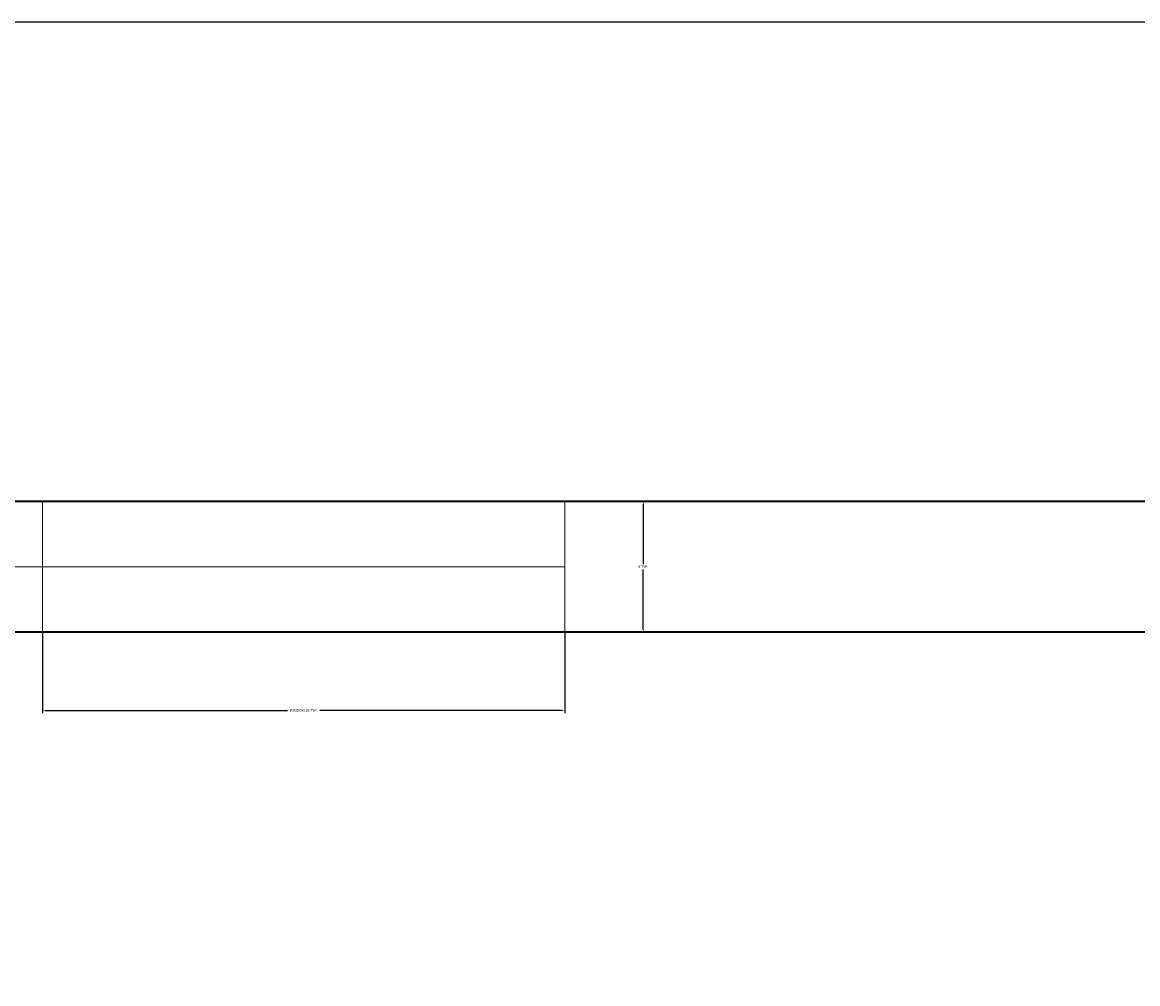
# Model space of a CAD drawing. Units: millimetres. Extents: x 27017497 to 27018854, y 7058029 to 7059154.
# Tile 46 of 91: x 27017673 to 27017750, y 7058557 to 7058623. Entities that reach past the tile are written whole.
import ezdxf

# ---------------------------------------------------------------- set-up
doc = ezdxf.new("R2010")
doc.units = ezdxf.units.MM
for name, color, linetype, lineweight in [('A-ANNO-DIMS', 2, 'Continuous', 18), ('A-GLAZ', 4, 'Continuous', 18), ('A-WALL', 7, 'Continuous', 35)]:
    doc.layers.add(name, color=color, linetype=linetype, lineweight=lineweight)
doc.styles.get("Standard").update_dxf_attribs({"font": 'arial.ttf'})
doc.dimstyles.get("Standard").update_dxf_attribs({"dimtxt": 0.18, "dimasz": 0.18, "dimexe": 0.18, "dimexo": 0.0625, "dimgap": 0.09, "dimtad": 0, "dimtih": 1, "dimtoh": 1, "dimdec": 4, "dimzin": 0, "dimdsep": 46, "dimtxsty": 'Standard', "dimcen": 0.09, "dimadec": 0, "dimazin": 0, "dimtfac": 1, "dimtdec": 4, "dimtofl": 0, "dimtmove": 0, "dimatfit": 3, "dimfxl": 1, "dimtolj": 1, "dimtzin": 0, "dimarcsym": 0})

# ---------------------------------------------------------------- blocks, each defined once
blk = doc.blocks.new('WINDOW-SINGLE-LIGHT')
blk.add_lwpolyline([(36, 4.5), (36, 0), (0, 0), (0, 9), (36, 9), (36, 4.5), (0, 4.5)])
blk = doc.blocks.new('*D19')
at = {"layer": 'A-ANNO-DIMS', "color": 0, "lineweight": -2, "transparency": 16777216}
for p, q in [((27017674.681, 7058580.826), (27017674.681, 7058575.309)), ((27017710.681, 7058580.826), (27017710.681, 7058575.309)), ((27017674.861, 7058575.489), (27017691.563, 7058575.489)), ((27017710.501, 7058575.489), (27017693.8, 7058575.489))]:
    blk.add_line(p, q, dxfattribs=at)
at = {"layer": 'A-ANNO-DIMS', "color": 0, "transparency": 16777216}
for points in [[(27017674.861, 7058575.519), (27017674.861, 7058575.459), (27017674.681, 7058575.489)], [(27017710.501, 7058575.519), (27017710.501, 7058575.459), (27017710.681, 7058575.489)]]:
    blk.add_solid(points, dxfattribs=at)
at = {"layer": 'Defpoints', "color": 0, "transparency": 16777216}
for p in [(27017674.681, 7058580.889), (27017710.681, 7058580.889), (27017710.681, 7058575.489)]:
    blk.add_point(p, dxfattribs=at)
at = {"layer": 'A-ANNO-DIMS', "color": 0, "transparency": 16777216, "insert": (27017692.681, 7058575.489), "char_height": 0.18, "attachment_point": 5}
blk.add_mtext('\\A1;WINDOW 36 TYP.', dxfattribs=at)
blk = doc.blocks.new('*D20')
at = {"layer": 'A-ANNO-DIMS', "color": 0, "lineweight": -2, "transparency": 16777216}
for p, q in [((27017710.744, 7058589.889), (27017716.261, 7058589.889)), ((27017716.081, 7058589.709), (27017716.081, 7058585.571)), ((27017716.081, 7058581.069), (27017716.081, 7058585.207)), ((27017710.744, 7058580.889), (27017716.261, 7058580.889))]:
    blk.add_line(p, q, dxfattribs=at)
at = {"layer": 'A-ANNO-DIMS', "color": 0, "transparency": 16777216}
for points in [[(27017716.051, 7058589.709), (27017716.111, 7058589.709), (27017716.081, 7058589.889)], [(27017716.051, 7058581.069), (27017716.111, 7058581.069), (27017716.081, 7058580.889)]]:
    blk.add_solid(points, dxfattribs=at)
at = {"layer": 'Defpoints', "color": 0, "transparency": 16777216}
for p in [(27017710.681, 7058589.889), (27017716.081, 7058589.889), (27017710.681, 7058580.889)]:
    blk.add_point(p, dxfattribs=at)
at = {"layer": 'A-ANNO-DIMS', "color": 0, "transparency": 16777216, "insert": (27017716.081, 7058585.389), "char_height": 0.18, "attachment_point": 5}
blk.add_mtext('\\A1;9 TYP.', dxfattribs=at)
blk = doc.blocks.new('*D48')
at = {"layer": 'A-ANNO-DIMS', "color": 0, "lineweight": -2, "transparency": 16777216}
for p, q in [((27018463.498, 7058622.912), (27017497.536, 7058622.912)), ((27017497.716, 7058622.732), (27017497.716, 7058357.753)), ((27017497.716, 7058092.41), (27017497.716, 7058357.389)), ((27018555.129, 7058092.23), (27017497.536, 7058092.23))]:
    blk.add_line(p, q, dxfattribs=at)
at = {"layer": 'A-ANNO-DIMS', "color": 0, "transparency": 16777216}
for points in [[(27017497.686, 7058622.732), (27017497.746, 7058622.732), (27017497.716, 7058622.912)], [(27017497.686, 7058092.41), (27017497.746, 7058092.41), (27017497.716, 7058092.23)]]:
    blk.add_solid(points, dxfattribs=at)
at = {"layer": 'Defpoints', "color": 0, "transparency": 16777216}
for p in [(27018463.561, 7058622.912), (27017497.716, 7058092.23), (27018555.192, 7058092.23)]:
    blk.add_point(p, dxfattribs=at)
at = {"layer": 'A-ANNO-DIMS', "color": 0, "transparency": 16777216, "insert": (27017497.716, 7058357.571), "char_height": 0.18, "attachment_point": 5}
blk.add_mtext('\\A1;530.7', dxfattribs=at)

msp = doc.modelspace()

# ---------------------------------------------------------------- linework, layer by layer
at = {"layer": 'A-WALL'}
for p, q in [((27017613.666, 7058589.912), (27018310.606, 7058589.912)), ((27017622.666, 7058580.912), (27018223.606, 7058580.912))]:
    msp.add_line(p, q, dxfattribs=at)

# ---------------------------------------------------------------- block references
at = {"layer": 'A-GLAZ'}
for p in [(27017638.686, 7058580.886), (27017674.681, 7058580.889)]:
    msp.add_blockref('WINDOW-SINGLE-LIGHT', p, dxfattribs=at)

# ---------------------------------------------------------------- dimensions: what is measured, and where the dimension line sits
at = {"layer": 'A-ANNO-DIMS'}
dim = msp.add_linear_dim(base=(27017497.716, 7058092.23), p1=(27018463.561, 7058622.912), p2=(27018555.192, 7058092.23), angle=90, dimstyle='Standard', override={"dimdec": 1, "dimlfac": 1, "dimrnd": 0, "dimzin": 0, "dimdsep": 46, "dimlunit": 2}, dxfattribs=at)
dim.commit()
dim.dimension.update_dxf_attribs({"geometry": '*D48', "text_midpoint": (27017497.716, 7058357.571)})
dim = msp.add_linear_dim(base=(27017716.081, 7058589.889), p1=(27017710.681, 7058580.889), p2=(27017710.681, 7058589.889), angle=90, text='<> TYP.', dimstyle='Standard', override={"dimdec": 0, "dimlfac": 1, "dimrnd": 0, "dimzin": 0, "dimdsep": 46, "dimlunit": 2}, dxfattribs=at)
dim.commit()
dim.dimension.update_dxf_attribs({"geometry": '*D20', "text_midpoint": (27017716.081, 7058585.389)})
dim = msp.add_linear_dim(base=(27017710.681, 7058575.489), p1=(27017674.681, 7058580.889), p2=(27017710.681, 7058580.889), text='WINDOW <> TYP.', dimstyle='Standard', override={"dimdec": 0, "dimlfac": 1, "dimrnd": 0, "dimzin": 0, "dimdsep": 46, "dimlunit": 2}, dxfattribs=at)
dim.commit()
dim.dimension.update_dxf_attribs({"geometry": '*D19', "text_midpoint": (27017692.681, 7058575.489)})

doc.saveas('drawing.dxf')
